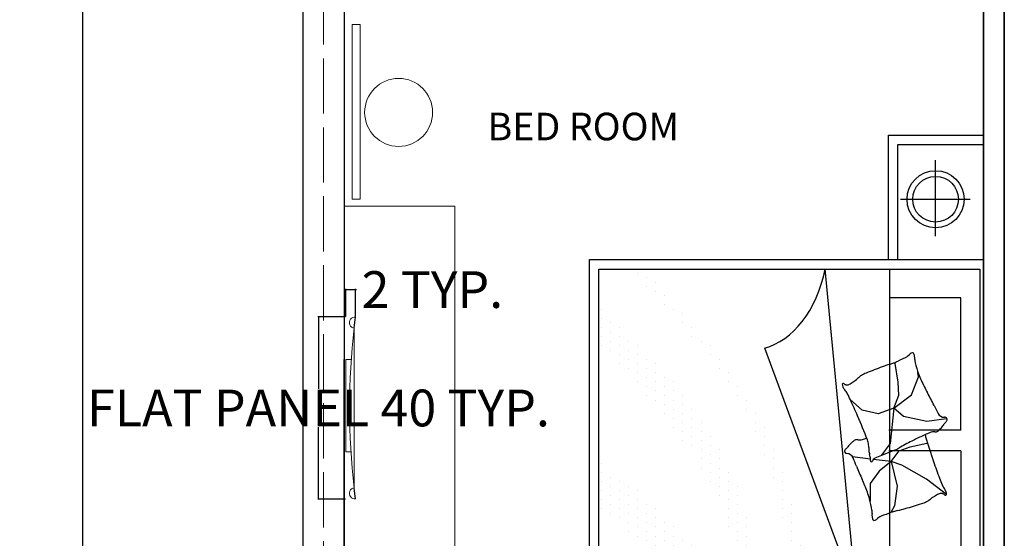
# Model space of a CAD drawing. Units: inches. Extents: x -48 to 50072, y 0 to 21068.
# Tile 65 of 75: x 697 to 911, y 803 to 915. Entities that reach past the tile are written whole.
import ezdxf

# ---------------------------------------------------------------- set-up
doc = ezdxf.new("R2010")
doc.units = ezdxf.units.IN
doc.header["$MEASUREMENT"] = 0
doc.linetypes.add('ACAD_ISO02W100', pattern=[15, 12, -3])
for name, color, linetype, lineweight in [('A-ANNO-DIMS', 2, 'Continuous', 18), ('A-AREA-IDEN', 7, 'Continuous', 18), ('A-EQPM', 8, 'Continuous', 18), ('A-FLOR-CASE', 9, 'Continuous', 18), ('A-WALL', 7, 'Continuous', 35), ('C-PROP', 7, 'Continuous', 25), ('C-PROP-REF', 32, 'ACAD_ISO02W100', 13), ('FURNITURE', 44, 'Continuous', 18)]:
    doc.layers.add(name, color=color, linetype=linetype, lineweight=lineweight)
doc.styles.get("Standard").update_dxf_attribs({"font": 'arial.ttf'})
doc.dimstyles.get("Standard").update_dxf_attribs({"dimtxt": 8, "dimasz": 0.18, "dimexe": 0.18, "dimexo": 0.0625, "dimgap": 0.09, "dimtad": 0, "dimtih": 1, "dimtoh": 1, "dimdec": 1, "dimzin": 0, "dimdsep": 46, "dimlunit": 4, "dimtxsty": 'Standard', "dimblk": 'ARCHTICK', "dimcen": 0.09, "dimadec": 0, "dimazin": 0, "dimtfac": 1, "dimtdec": 1, "dimtofl": 0, "dimtmove": 0, "dimatfit": 3, "dimldrblk": 'ARCHTICK', "dimfxl": 1, "dimtolj": 1, "dimtzin": 0, "dimarcsym": 0})

# ---------------------------------------------------------------- blocks, each defined once
blk = doc.blocks.new('nhrygfdu7yu')
at = {"layer": 'Defpoints'}
for p, q in [((1019.17, 828.61), (845.97, 828.61)), ((845.97, 801.61), (845.97, 828.61)), ((848.67, 804.31), (848.67, 828.61)), ((881.27, 716.83), (881.27, 828.61)), ((884.03, 719.53), (884.03, 827.53)), ((884.03, 827.53), (981.17, 827.53)), ((981.17, 827.53), (981.17, 719.53)), ((983.87, 828.61), (983.87, 716.83)), ((1016.47, 804.31), (1016.47, 828.61)), ((1019.17, 801.61), (1019.17, 828.61)), ((864.18, 805.04), (864.18, 824.84)), ((1000.24, 805.98), (1000.24, 825.78)), ((892.12, 822.13), (892.12, 801.97)), ((929.67, 822.13), (892.12, 822.13)), ((929.67, 822.13), (929.67, 801.78)), ((935.52, 822.13), (935.52, 801.78)), ((935.52, 822.13), (973.07, 822.13)), ((973.07, 822.13), (973.07, 801.97)), ((926.47, 818.07), (927.21, 812.5)), ((947.88, 818.06), (943.61, 812.45)), ((1010.72, 815.93), (989.15, 815.93)), ((874.65, 814.99), (853.09, 814.99)), ((927.21, 812.5), (925.82, 805.91)), ((934.43, 807.75), (933.36, 812.55)), ((943.61, 812.45), (939.55, 805.41)), ((914.58, 810.18), (913.28, 809.99)), ((919.69, 808.14), (914.58, 810.18)), ((923.4, 803.12), (919.69, 808.14)), ((935.49, 804.66), (934.43, 807.75)), ((881.07, 804.31), (848.67, 804.31)), ((881.07, 804.31), (881.07, 804.31)), ((916.07, 804.42), (910.77, 803.49)), ((919.78, 804.61), (916.07, 804.42)), ((923.4, 803.12), (919.78, 804.61)), ((925.82, 805.91), (923.4, 803.12)), ((938.59, 802.42), (935.49, 804.66)), ((939.55, 805.41), (938.59, 802.42)), ((938.59, 802.42), (945.53, 804.13)), ((945.53, 804.13), (951.08, 803.38)), ((984.07, 804.31), (1016.47, 804.31)), ((984.07, 804.31), (984.07, 804.31)), ((881.07, 801.61), (845.97, 801.61)), ((884.06, 801.97), (981.18, 801.97)), ((910.77, 803.49), (910.59, 803.15)), ((923.4, 803.12), (925.08, 798.67)), ((923.4, 803.12), (933.44, 802.1)), ((933.44, 802.1), (936.13, 800.15)), ((935.45, 803.17), (936.69, 800.13)), ((938.59, 802.42), (937.95, 797.34)), ((938.59, 802.42), (941.26, 799.01)), ((951.08, 803.38), (953.02, 802.3)), ((984.07, 801.61), (1019.17, 801.61)), ((925.08, 798.67), (923.96, 794.21)), ((936.13, 800.15), (936.78, 799.69)), ((936.69, 800.13), (937.65, 797.78)), ((941.26, 799.01), (944.78, 796.45)), ((937.86, 796.54), (937.22, 791.44)), ((944.78, 796.45), (949.8, 796.45)), ((981.13, 793.06), (883.98, 783.7)), ((923.96, 794.21), (921.07, 790.83)), ((906.36, 766.47), (977.44, 792.73)), ((976.41, 779.36), (976.41, 779.36)), ((978.98, 779.36), (978.98, 779.36)), ((962.27, 776.79), (962.27, 776.79)), ((964.84, 776.79), (964.84, 776.79)), ((967.41, 776.79), (967.41, 776.79)), ((969.98, 776.79), (969.98, 776.79)), ((972.55, 776.79), (972.55, 776.79)), ((975.13, 776.79), (975.13, 776.79)), ((977.7, 776.79), (977.7, 776.79)), ((980.27, 776.79), (980.27, 776.79)), ((950.69, 774.21), (950.69, 774.21)), ((953.27, 774.21), (953.27, 774.21)), ((955.84, 774.21), (955.84, 774.21)), ((958.41, 774.21), (958.41, 774.21)), ((960.98, 774.21), (960.98, 774.21)), ((963.55, 774.21), (963.55, 774.21)), ((966.13, 774.21), (966.13, 774.21)), ((968.7, 774.21), (968.7, 774.21)), ((941.69, 771.64), (941.69, 771.64)), ((944.27, 771.64), (944.27, 771.64)), ((946.84, 771.64), (946.84, 771.64)), ((949.41, 771.64), (949.41, 771.64)), ((951.98, 771.64), (951.98, 771.64)), ((954.55, 771.64), (954.55, 771.64)), ((935.26, 769.07), (935.26, 769.07)), ((937.84, 769.07), (937.84, 769.07)), ((940.41, 769.07), (940.41, 769.07)), ((942.98, 769.07), (942.98, 769.07)), ((928.83, 766.5), (928.83, 766.5)), ((931.41, 766.5), (931.41, 766.5)), ((933.98, 766.5), (933.98, 766.5)), ((936.55, 766.5), (936.55, 766.5)), ((975.13, 766.5), (975.13, 766.5)), ((977.7, 766.5), (977.7, 766.5)), ((980.27, 766.5), (980.27, 766.5)), ((924.98, 763.93), (924.98, 763.93)), ((927.55, 763.93), (927.55, 763.93)), ((930.12, 763.93), (930.12, 763.93)), ((963.55, 763.93), (963.55, 763.93)), ((966.13, 763.93), (966.13, 763.93)), ((968.7, 763.93), (968.7, 763.93)), ((971.27, 763.93), (971.27, 763.93)), ((973.84, 763.93), (973.84, 763.93)), ((976.41, 763.93), (976.41, 763.93)), ((978.98, 763.93), (978.98, 763.93)), ((921.12, 761.35), (921.12, 761.35)), ((923.69, 761.35), (923.69, 761.35)), ((954.55, 761.35), (954.55, 761.35)), ((957.12, 761.35), (957.12, 761.35)), ((959.7, 761.35), (959.7, 761.35)), ((962.27, 761.35), (962.27, 761.35)), ((964.84, 761.35), (964.84, 761.35)), ((967.41, 761.35), (967.41, 761.35)), ((969.98, 761.35), (969.98, 761.35)), ((972.55, 761.35), (972.55, 761.35)), ((975.13, 761.35), (975.13, 761.35)), ((917.26, 758.78), (917.26, 758.78)), ((919.83, 758.78), (919.83, 758.78)), ((945.55, 758.78), (945.55, 758.78)), ((948.12, 758.78), (948.12, 758.78)), ((950.69, 758.78), (950.69, 758.78)), ((953.27, 758.78), (953.27, 758.78)), ((955.84, 758.78), (955.84, 758.78)), ((958.41, 758.78), (958.41, 758.78)), ((960.98, 758.78), (960.98, 758.78)), ((963.55, 758.78), (963.55, 758.78)), ((913.4, 756.21), (913.4, 756.21)), ((915.98, 756.21), (915.98, 756.21)), ((941.69, 756.21), (941.69, 756.21)), ((944.27, 756.21), (944.27, 756.21)), ((946.84, 756.21), (946.84, 756.21)), ((949.41, 756.21), (949.41, 756.21)), ((951.98, 756.21), (951.98, 756.21)), ((954.55, 756.21), (954.55, 756.21)), ((957.12, 756.21), (957.12, 756.21)), ((980.27, 756.21), (980.27, 756.21)), ((905.69, 751.07), (905.69, 751.07)), ((908.26, 751.07), (908.26, 751.07)), ((909.55, 753.64), (909.55, 753.64)), ((912.12, 753.64), (912.12, 753.64)), ((931.41, 751.07), (931.41, 751.07)), ((933.98, 751.07), (933.98, 751.07)), ((935.26, 753.64), (935.26, 753.64)), ((936.55, 751.07), (936.55, 751.07)), ((937.84, 753.64), (937.84, 753.64)), ((939.12, 751.07), (939.12, 751.07)), ((940.41, 753.64), (940.41, 753.64)), ((941.69, 751.07), (941.69, 751.07)), ((942.98, 753.64), (942.98, 753.64)), ((944.27, 751.07), (944.27, 751.07)), ((945.55, 753.64), (945.55, 753.64)), ((948.12, 753.64), (948.12, 753.64)), ((969.98, 751.07), (969.98, 751.07)), ((972.55, 751.07), (972.55, 751.07)), ((975.13, 751.07), (975.13, 751.07)), ((976.41, 753.64), (976.41, 753.64)), ((977.7, 751.07), (977.7, 751.07)), ((978.98, 753.64), (978.98, 753.64)), ((980.27, 751.07), (980.27, 751.07)), ((904.4, 748.5), (904.4, 748.5)), ((927.55, 748.5), (927.55, 748.5)), ((930.12, 748.5), (930.12, 748.5)), ((932.69, 748.5), (932.69, 748.5)), ((935.26, 748.5), (935.26, 748.5)), ((937.84, 748.5), (937.84, 748.5)), ((940.41, 748.5), (940.41, 748.5)), ((966.13, 748.5), (966.13, 748.5)), ((968.7, 748.5), (968.7, 748.5)), ((971.27, 748.5), (971.27, 748.5)), ((973.84, 748.5), (973.84, 748.5)), ((976.41, 748.5), (976.41, 748.5)), ((978.98, 748.5), (978.98, 748.5)), ((900.55, 745.92), (900.55, 745.92)), ((903.12, 745.92), (903.12, 745.92)), ((923.69, 745.92), (923.69, 745.92)), ((926.26, 745.92), (926.26, 745.92)), ((928.83, 745.92), (928.83, 745.92)), ((931.41, 745.92), (931.41, 745.92)), ((933.98, 745.92), (933.98, 745.92)), ((962.27, 745.92), (962.27, 745.92)), ((964.84, 745.92), (964.84, 745.92)), ((967.41, 745.92), (967.41, 745.92)), ((969.98, 745.92), (969.98, 745.92)), ((972.55, 745.92), (972.55, 745.92)), ((975.13, 745.92), (975.13, 745.92)), ((977.7, 745.92), (977.7, 745.92)), ((896.69, 743.35), (896.69, 743.35)), ((899.26, 743.35), (899.26, 743.35)), ((919.83, 743.35), (919.83, 743.35)), ((922.41, 743.35), (922.41, 743.35)), ((924.98, 743.35), (924.98, 743.35)), ((927.55, 743.35), (927.55, 743.35)), ((930.12, 743.35), (930.12, 743.35)), ((932.69, 743.35), (932.69, 743.35)), ((960.98, 743.35), (960.98, 743.35)), ((963.55, 743.35), (963.55, 743.35)), ((966.13, 743.35), (966.13, 743.35)), ((968.7, 743.35), (968.7, 743.35)), ((971.27, 743.35), (971.27, 743.35)), ((973.84, 743.35), (973.84, 743.35)), ((895.4, 740.78), (895.4, 740.78)), ((915.98, 740.78), (915.98, 740.78)), ((918.55, 740.78), (918.55, 740.78)), ((921.12, 740.78), (921.12, 740.78)), ((923.69, 740.78), (923.69, 740.78)), ((926.26, 740.78), (926.26, 740.78)), ((928.83, 740.78), (928.83, 740.78)), ((957.12, 740.78), (957.12, 740.78)), ((959.7, 740.78), (959.7, 740.78)), ((962.27, 740.78), (962.27, 740.78)), ((964.84, 740.78), (964.84, 740.78)), ((967.41, 740.78), (967.41, 740.78)), ((969.98, 740.78), (969.98, 740.78)), ((891.54, 738.21), (891.54, 738.21)), ((894.12, 738.21), (894.12, 738.21)), ((914.69, 738.21), (914.69, 738.21)), ((917.26, 738.21), (917.26, 738.21)), ((919.83, 738.21), (919.83, 738.21)), ((922.41, 738.21), (922.41, 738.21)), ((924.98, 738.21), (924.98, 738.21)), ((955.84, 738.21), (955.84, 738.21)), ((958.41, 738.21), (958.41, 738.21)), ((960.98, 738.21), (960.98, 738.21)), ((963.55, 738.21), (963.55, 738.21)), ((966.13, 738.21), (966.13, 738.21)), ((887.69, 735.64), (887.69, 735.64)), ((890.26, 735.64), (890.26, 735.64)), ((910.83, 735.64), (910.83, 735.64)), ((913.4, 735.64), (913.4, 735.64)), ((915.98, 735.64), (915.98, 735.64)), ((918.55, 735.64), (918.55, 735.64)), ((921.12, 735.64), (921.12, 735.64)), ((951.98, 735.64), (951.98, 735.64)), ((954.55, 735.64), (954.55, 735.64)), ((957.12, 735.64), (957.12, 735.64)), ((959.7, 735.64), (959.7, 735.64)), ((962.27, 735.64), (962.27, 735.64)), ((964.84, 735.64), (964.84, 735.64)), ((886.4, 733.07), (886.4, 733.07)), ((888.97, 733.07), (888.97, 733.07)), ((909.55, 733.07), (909.55, 733.07)), ((912.12, 733.07), (912.12, 733.07)), ((914.69, 733.07), (914.69, 733.07)), ((917.26, 733.07), (917.26, 733.07)), ((919.83, 733.07), (919.83, 733.07)), ((950.69, 733.07), (950.69, 733.07)), ((953.27, 733.07), (953.27, 733.07)), ((955.84, 733.07), (955.84, 733.07)), ((958.41, 733.07), (958.41, 733.07)), ((960.98, 733.07), (960.98, 733.07)), ((885.12, 730.49), (885.12, 730.49)), ((905.69, 730.49), (905.69, 730.49)), ((908.26, 730.49), (908.26, 730.49)), ((910.83, 730.49), (910.83, 730.49)), ((913.4, 730.49), (913.4, 730.49)), ((915.98, 730.49), (915.98, 730.49)), ((946.84, 730.49), (946.84, 730.49)), ((949.41, 730.49), (949.41, 730.49)), ((951.98, 730.49), (951.98, 730.49)), ((954.55, 730.49), (954.55, 730.49)), ((957.12, 730.49), (957.12, 730.49)), ((959.7, 730.49), (959.7, 730.49)), ((904.4, 727.92), (904.4, 727.92)), ((906.97, 727.92), (906.97, 727.92)), ((909.55, 727.92), (909.55, 727.92)), ((912.12, 727.92), (912.12, 727.92)), ((945.55, 727.92), (945.55, 727.92)), ((948.12, 727.92), (948.12, 727.92)), ((950.69, 727.92), (950.69, 727.92)), ((953.27, 727.92), (953.27, 727.92)), ((955.84, 727.92), (955.84, 727.92)), ((958.41, 727.92), (958.41, 727.92)), ((900.55, 725.35), (900.55, 725.35)), ((903.12, 725.35), (903.12, 725.35)), ((905.69, 725.35), (905.69, 725.35)), ((908.26, 725.35), (908.26, 725.35)), ((910.83, 725.35), (910.83, 725.35)), ((944.27, 725.35), (944.27, 725.35)), ((946.84, 725.35), (946.84, 725.35)), ((949.41, 725.35), (949.41, 725.35)), ((951.98, 725.35), (951.98, 725.35)), ((954.55, 725.35), (954.55, 725.35)), ((895.4, 720.21), (895.4, 720.21)), ((897.97, 720.21), (897.97, 720.21)), ((899.26, 722.78), (899.26, 722.78)), ((900.55, 720.21), (900.55, 720.21)), ((901.83, 722.78), (901.83, 722.78)), ((903.12, 720.21), (903.12, 720.21)), ((904.4, 722.78), (904.4, 722.78)), ((905.69, 720.21), (905.69, 720.21)), ((906.97, 722.78), (906.97, 722.78)), ((939.12, 720.21), (939.12, 720.21)), ((941.69, 720.21), (941.69, 720.21)), ((942.98, 722.78), (942.98, 722.78)), ((944.27, 720.21), (944.27, 720.21)), ((945.55, 722.78), (945.55, 722.78)), ((946.84, 720.21), (946.84, 720.21)), ((948.12, 722.78), (948.12, 722.78)), ((949.41, 720.21), (949.41, 720.21)), ((950.69, 722.78), (950.69, 722.78)), ((951.98, 720.21), (951.98, 720.21)), ((953.27, 722.78), (953.27, 722.78)), ((981.17, 719.53), (884.03, 719.53)), ((983.87, 716.83), (881.27, 716.83))]:
    blk.add_line(p, q, dxfattribs=at)
for centre, radius in [((1000.24, 815.93), 8.1), ((864.18, 814.99), 8.1), ((864.18, 814.99), 6.48), ((1000.24, 815.93), 6.48)]:
    blk.add_circle(centre, radius, dxfattribs=at)
for centre, radius, start, end in [((926.67, 817.58), 0.687, 51.1864, 183.2455), ((924.75, 815.18), 3.76, 45.8726, 51.1864), ((948.22, 814.9), 3.25, 110.3452, 128.5854), ((947.75, 816.16), 1.9, 86.0516, 110.3452), ((947.87, 817.82), 0.239, 13.2808, 86.0516), ((848.26, 964.34), 167.25, 296.4147, 297.2902), ((924.05, 817.43), 1.94, 297.2902, 3.2455), ((929.07, 819.63), 2.44, 225.8726, 232.4713), ((940.16, 834.08), 20.66, 232.4713, 233.7837), ((906.88, 788.64), 35.67, 52.7849, 53.7837), ((921.35, 807.68), 11.75, 46.4776, 52.7849), ((926.56, 813.17), 4.18, 35.8936, 46.4776), ((928.96, 814.91), 1.22, 351.9508, 35.8936), ((848.62, 1074.38), 275.09, 289.0836, 290.1287), ((927.73, 858.54), 45.2, 290.1287, 292.7069), ((943.53, 820.78), 4.28, 292.7069, 308.5854), ((951.77, 816.3), 4.17, 169.5926, 177.2714), ((948.44, 816.46), 0.826, 177.2714, 194.5709), ((949.69, 816.78), 2.12, 194.5709, 206.8179), ((948.43, 816.91), 0.765, 126.5792, 169.5926), ((964.76, 824.4), 19.01, 206.8179, 210.9056), ((947.77, 817.8), 0.34, 306.5792, 13.2808), ((771.78, 1091.44), 315.27, 297.4921, 297.8482), ((1072.97, 521.35), 329.5, 117.4999, 117.8482), ((971.1, 717.04), 108.88, 116.4147, 117.4999), ((932.62, 814.39), 2.47, 171.9508, 202.4162), ((980.52, 834.15), 54.29, 202.4162, 205.0529), ((883.03, 974.91), 169.83, 286.6085, 289.0836), ((957.44, 820.02), 10.47, 210.9056, 219.7005), ((946.01, 810.53), 4.37, 26.0735, 39.7005), ((940.41, 807.79), 10.61, 17.8396, 26.0735), ((905.47, 831.87), 23.22, 282.6252, 290.7486), ((901.77, 841.65), 33.68, 290.7486, 297.4921), ((929.77, 818.2), 6.29, 280.7366, 286.6085), ((1013.86, 849.73), 91.09, 205.0529, 207.0884), ((847.55, 777.91), 108.16, 15.2625, 17.8396), ((908.02, 808.45), 0.313, 121.6917, 179.0386), ((908.61, 808.44), 0.905, 179.0386, 229.4914), ((909.3, 806.38), 2.75, 103.0402, 121.6917), ((905.38, 804.66), 4.08, 26.3332, 49.4914), ((909.41, 805.91), 3.23, 86.6119, 103.0402), ((909.8, 812.53), 3.4, 266.6119, 282.6252), ((1008.01, 846.74), 84.52, 207.0884, 209.936), ((780.21, 742.7), 143.74, 25.1732, 26.3332), ((924.73, 798.79), 11.57, 22.2355, 29.936), ((866.04, 782.95), 89, 13.841, 15.2625), ((981.05, 811.29), 29.45, 193.841, 196.3122), ((901.51, 799.71), 9.71, 20.7081, 25.1732), ((883.04, 792.73), 29.45, 18.2369, 20.7081), ((995.54, 829.8), 89, 198.2369, 199.6584), ((962.1, 805.74), 9.71, 196.3122, 200.7773), ((1087.42, 853.29), 143.74, 200.7773, 201.9373), ((1013.59, 836.25), 108.16, 199.6584, 202.2355), ((957.87, 801.11), 4.08, 201.9373, 225.0955), ((993.31, 637.11), 169.83, 111.0043, 113.4795), ((934.7, 789.77), 6.29, 98.1216, 111.0043), ((934.31, 792.46), 3.58, 85.4882, 98.1216), ((934.9, 799.87), 3.85, 265.4882, 277.6784), ((934.12, 805.65), 9.69, 277.6784, 284.8807), ((939.32, 786.09), 10.56, 97.9822, 104.8807), ((938.8, 798.25), 1.24, 202.2355, 252.8133), ((938.1, 794.73), 1.83, 85.7407, 97.9822), ((938.28, 797.05), 0.497, 265.7407, 289.3799), ((938.36, 796.82), 0.252, 289.3799, 72.8133), ((958.63, 763.95), 33.68, 106.3527, 113.0962), ((955.69, 773.98), 23.22, 98.2293, 106.3527), ((952.85, 793.6), 3.4, 82.216, 98.2293), ((953.75, 800.17), 3.23, 262.216, 278.6443), ((953.82, 799.69), 2.75, 278.6443, 297.2959), ((954.35, 797.58), 0.905, 354.6428, 45.0955), ((954.94, 797.53), 0.313, 297.2959, 354.6428), ((923.29, 799.33), 10.61, 202.2355, 210.4694), ((917.92, 796.17), 4.37, 210.4694, 224.0964), ((907.26, 785.84), 10.47, 35.3015, 44.0964), ((1035.25, 540.56), 275.09, 113.4795, 114.5246), ((880.68, 777.46), 54.29, 18.0203, 19.3448), ((929.96, 793.49), 2.47, 347.5549, 18.0203), ((933.57, 792.7), 1.22, 167.5549, 211.4977), ((899.06, 893.51), 108.88, 292.0188, 293.104), ((812.48, 1096.43), 329.5, 293.104, 293.4523), ((1069.09, 504.93), 315.27, 113.0962, 113.4523), ((900.29, 780.91), 19.01, 31.2138, 35.3015), ((914.73, 789.66), 2.12, 18.9668, 31.2138), ((915.96, 790.08), 0.826, 1.6673, 18.9668), ((912.62, 789.98), 4.17, 353.9885, 1.6673), ((939.83, 749.71), 45.2, 114.5246, 117.1028), ((936.09, 794.24), 4.18, 211.4977, 222.0817), ((941.71, 799.32), 11.75, 222.0817, 228.389), ((957.59, 817.2), 35.67, 228.389, 229.3878), ((920.93, 774.44), 20.66, 48.0754, 49.3878), ((938.27, 789.81), 1.94, 112.8944, 178.8496), ((1002.58, 637.52), 167.25, 112.0188, 112.8944), ((916.73, 788.79), 0.34, 130.9751, 197.6767), ((916.63, 788.76), 0.239, 197.6767, 270.4475), ((916, 789.63), 0.765, 310.9751, 353.9885), ((916.62, 790.42), 1.9, 270.4475, 294.7411), ((916.05, 791.65), 3.25, 294.7411, 312.9813), ((921.18, 786.14), 4.28, 117.1028, 132.9813), ((933.1, 787.99), 2.44, 41.4767, 48.0754), ((937.75, 792.1), 3.76, 221.4767, 226.7905), ((935.64, 789.86), 0.687, 226.7905, 358.8496)]:
    blk.add_arc(centre, radius, start, end, dxfattribs=at)
blk.add_ellipse((874.1, 762.91), major_axis=(32.71, 0), ratio=0.667085, start_param=0.16392, end_param=1.263761, dxfattribs=at)
blk = doc.blocks.new('DISPLAY-FLAT-PANEL')
for p, q in [((1.73, 37.17), (2.01, 39.54)), ((1.83, 37.19), (2.11, 39.53)), ((1.83, 2.35), (1.83, 37.19)), ((1.83, 37.19), (1.83, 37.19)), ((1.2, 30.3), (0, 30.3)), ((0, 30.3), (0, 10.23)), ((0, 10.23), (1.13, 10.23)), ((1.73, 2.37), (2.01, 0)), ((1.83, 2.35), (2.11, 0.01))]:
    blk.add_line(p, q)
for centre, radius, start, end in [((1.97, 38.34), 1.2, 83.3215, 263.5313), ((153.03, 19.77), 152.2, 173.4285, 186.5715), ((1.97, 1.2), 1.2, 96.4687, 276.6785)]:
    blk.add_arc(centre, radius, start, end)
blk = doc.blocks.new('_ArchTick')
at = {"color": 0, "linetype": 'ByBlock', "const_width": 0.15}
blk.add_lwpolyline([(-0.5, -0.5), (0.5, 0.5)], dxfattribs=at)
blk = doc.blocks.new('*D84')
at = {"layer": 'A-ANNO-DIMS', "color": 0, "lineweight": -2, "transparency": 16777216}
for p, q in [((768.04, 850.74), (761.97, 850.74)), ((762.15, 850.74), (762.15, 835.1)), ((762.15, 811.11), (762.15, 826.75)), ((768.04, 811.11), (761.97, 811.11))]:
    blk.add_line(p, q, dxfattribs=at)
at = {"layer": 'Defpoints', "color": 0, "transparency": 16777216}
for p in [(762.15, 850.74), (768.1, 850.74), (768.1, 811.11)]:
    blk.add_point(p, dxfattribs=at)
at = {"layer": 'A-ANNO-DIMS', "color": 0, "lineweight": -2, "transparency": 16777216, "xscale": 0.18, "yscale": 0.18, "zscale": 0.18}
for p, rotation in [((762.15, 850.74), 90), ((762.15, 811.11), 270)]:
    blk.add_blockref('_ArchTick', p, dxfattribs=dict(at, rotation=rotation))
at = {"layer": 'A-ANNO-DIMS', "color": 0, "transparency": 16777216, "insert": (762.15, 830.93), "char_height": 8, "attachment_point": 5}
blk.add_mtext('\\A1;FLAT PANEL 40 TYP.', dxfattribs=at)
blk = doc.blocks.new('*D85')
at = {"layer": 'A-ANNO-DIMS', "color": 0, "lineweight": -2, "transparency": 16777216}
for p, q in [((768.1, 850.8), (768.1, 856.86)), ((768.1, 856.68), (770.21, 856.68)), ((770.21, 850.8), (770.21, 856.86)), ((770.21, 856.68), (770.39, 856.68))]:
    blk.add_line(p, q, dxfattribs=at)
at = {"layer": 'Defpoints', "color": 0, "transparency": 16777216}
for p in [(770.21, 856.68), (768.1, 850.74), (770.21, 850.74)]:
    blk.add_point(p, dxfattribs=at)
at = {"layer": 'A-ANNO-DIMS', "color": 0, "lineweight": -2, "transparency": 16777216, "xscale": 0.18, "yscale": 0.18, "zscale": 0.18, "rotation": 180}
blk.add_blockref('_ArchTick', (768.1, 856.68), dxfattribs=at)
at = {"layer": 'A-ANNO-DIMS', "color": 0, "lineweight": -2, "transparency": 16777216, "xscale": 0.18, "yscale": 0.18, "zscale": 0.18}
blk.add_blockref('_ArchTick', (770.21, 856.68), dxfattribs=at)
at = {"layer": 'A-ANNO-DIMS', "color": 0, "transparency": 16777216, "insert": (786.91, 856.68), "char_height": 8, "attachment_point": 5}
blk.add_mtext('\\A1;2 TYP.', dxfattribs=at)
blk = doc.blocks.new('*D130')
at = {"layer": 'A-ANNO-DIMS', "color": 0, "lineweight": -2, "transparency": 16777216}
for p, q in [((758.7, 1241.46), (710.63, 1241.46)), ((710.81, 1241.46), (710.81, 767.29)), ((710.81, 284.76), (710.81, 758.94)), ((758.7, 284.76), (710.63, 284.76))]:
    blk.add_line(p, q, dxfattribs=at)
at = {"layer": 'Defpoints', "color": 0, "transparency": 16777216}
for p in [(710.81, 1241.46), (758.76, 1241.46), (758.76, 284.76)]:
    blk.add_point(p, dxfattribs=at)
at = {"layer": 'A-ANNO-DIMS', "color": 0, "lineweight": -2, "transparency": 16777216, "xscale": 0.18, "yscale": 0.18, "zscale": 0.18}
for p, rotation in [((710.81, 1241.46), 90), ((710.81, 284.76), 270)]:
    blk.add_blockref('_ArchTick', p, dxfattribs=dict(at, rotation=rotation))
at = {"layer": 'A-ANNO-DIMS', "color": 0, "transparency": 16777216, "insert": (710.81, 763.11), "char_height": 8, "attachment_point": 5}
blk.add_mtext('\\A1;956.7', dxfattribs=at)

msp = doc.modelspace()

# ---------------------------------------------------------------- linework, layer by layer
at = {"layer": 'A-FLOR-CASE'}
for p, q in [((791.761, 874.822), (767.761, 874.822)), ((791.761, 757.464), (791.761, 874.822))]:
    msp.add_line(p, q, dxfattribs=at)
at = {"layer": 'A-WALL'}
for p, q in [((906.761, 931.464), (906.761, 757.464)), ((911.261, 931.464), (911.261, 748.464)), ((767.761, 757.464), (767.761, 841.464))]:
    msp.add_line(p, q, dxfattribs=at)
at = {"layer": 'C-PROP'}
for p, q in [((758.761, 1241.464), (758.761, 284.764)), ((767.761, 931.464), (767.761, 293.764))]:
    msp.add_line(p, q, dxfattribs=at)
at = {"layer": 'C-PROP-REF'}
msp.add_line((763.261, 1236.964), (763.261, 284.764), dxfattribs=at)
at = {"layer": 'FURNITURE'}
msp.add_lwpolyline([(769.448, 914.302), (771.236, 914.302), (771.236, 876.342), (769.448, 876.342)], close=True, dxfattribs=at)
msp.add_circle((779.576, 895.211), 7.394, dxfattribs=at)

# ---------------------------------------------------------------- block references
at = {"layer": 'A-EQPM'}
msp.add_blockref('DISPLAY-FLAT-PANEL', (768.098, 811.156), dxfattribs=at)
at = {"layer": 'FURNITURE', "xscale": 0.7669307891904348, "yscale": 0.7669307891904348, "zscale": 0.7669307891904348, "rotation": 270}
msp.add_blockref('nhrygfdu7yu', (271.278, 1539.095), dxfattribs=at)

# ---------------------------------------------------------------- texts
at = {"layer": 'A-AREA-IDEN', "insert": (798.895, 895.145), "char_height": 6, "attachment_point": 1}
msp.add_mtext_dynamic_manual_height_columns('BED ROOM ', width=57.4792, gutter_width=30, heights=[0], dxfattribs=at)

# ---------------------------------------------------------------- dimensions: what is measured, and where the dimension line sits
at = {"layer": 'A-ANNO-DIMS'}
dim = msp.add_linear_dim(base=(710.811, 1241.464), p1=(758.761, 284.764), p2=(758.761, 1241.464), angle=90, dimstyle='Standard', override={"dimdec": 1, "dimlfac": 1, "dimrnd": 0, "dimzin": 0, "dimdsep": 46, "dimlunit": 2}, dxfattribs=at)
dim.commit()
dim.dimension.update_dxf_attribs({"geometry": '*D130', "text_midpoint": (710.811, 763.114)})
dim = msp.add_linear_dim(base=(770.205, 856.68), p1=(768.098, 850.737), p2=(770.205, 850.737), text='<> TYP.', dimstyle='Standard', override={"dimdec": 0, "dimlfac": 1, "dimrnd": 0, "dimzin": 0, "dimdsep": 46, "dimlunit": 2}, dxfattribs=at)
dim.commit()
dim.dimension.update_dxf_attribs({"geometry": '*D85', "text_midpoint": (786.906, 856.68)})
dim = msp.add_linear_dim(base=(762.154, 850.737), p1=(768.098, 811.114), p2=(768.098, 850.737), angle=90, text='FLAT PANEL <> TYP.', dimstyle='Standard', override={"dimdec": 0, "dimlfac": 1, "dimrnd": 0, "dimzin": 0, "dimdsep": 46, "dimlunit": 2}, dxfattribs=at)
dim.commit()
dim.dimension.update_dxf_attribs({"geometry": '*D84', "text_midpoint": (762.154, 830.926)})

doc.saveas('drawing.dxf')
